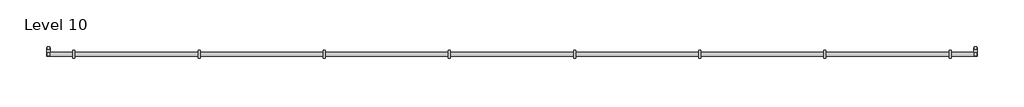
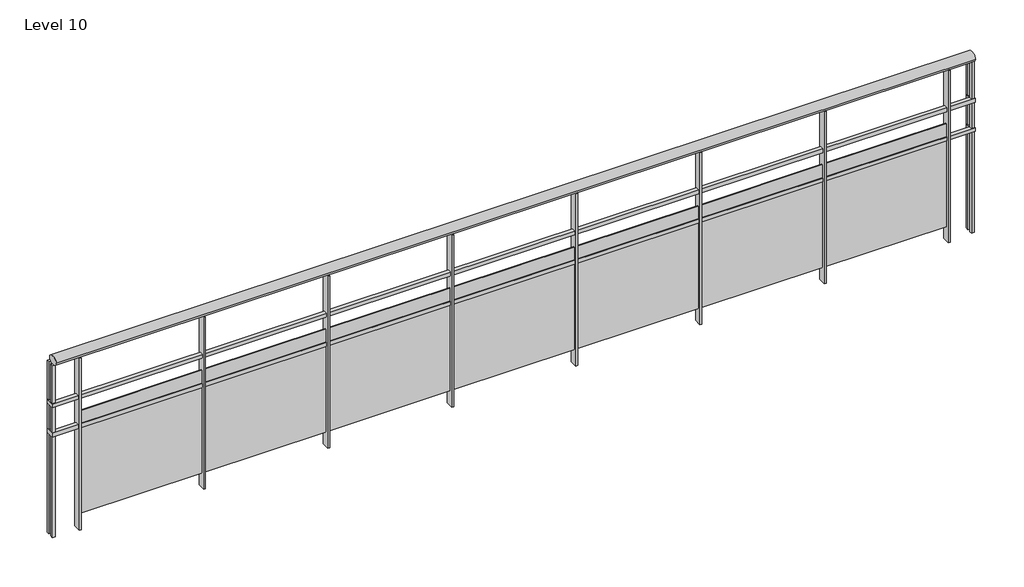
# One storey: 1 railing.
"""IFC4 building model written with IfcOpenShell, lengths in millimetres."""

from ifc_helpers import new_model, si_unit, point, frame, origin, place, context, project, spatial, polyline, ellipse_curve, trimmed, outline, extrude, faceted_brep, element, save
from ifc_brep_helpers import plane_surface, extruded_surface, advanced_brep

model = new_model("IFC4")

# Units and contexts
model_context = context("Model", 3, world=origin())
ifc_project = project(units=[si_unit("LENGTHUNIT", "METRE", prefix="MILLI")], contexts=[model_context])

# Site, building, storey
site = spatial("IfcSite", under=ifc_project)
building = spatial("IfcBuilding", under=site)
storey = spatial("IfcBuildingStorey", under=building, Name="Level 10", Elevation=19812.0)

# Railing
placement = place(None, origin())
element("IfcRailing", 1, ObjectType="Glass Panel - Bottom Fill", at=placement, inside=storey, context=model_context, shape_type="SolidModel", body=[
    advanced_brep(
    [(-17715.2963079, -4526.0757947, 21031.2), (-17715.2963079, -4449.8757947, 21031.2), (-23735.0963079, -4526.0757947, 21031.2), (-23735.0963079, -4449.8757947, 21031.2)],
    [
        (0, 1, ellipse_curve(frame((-17715.2963079, -4487.9757947, 21031.2), z_axis=(1.0, 0.0, 0.0), x_axis=(0.0, 1.0, 0.0)), 38.1, 28.575)),
        (1, 0, ellipse_curve(frame((-17715.2963079, -4487.9757947, 21031.2), z_axis=(1.0, 0.0, 0.0), x_axis=(0.0, 1.0, 0.0)), 38.1, 28.575)),
        (2, 3, ellipse_curve(frame((-23735.0963079, -4487.9757947, 21031.2), z_axis=(-1.0, 0.0, 0.0), x_axis=(0.0, 1.0, 0.0)), 38.1, 28.575)),
        (3, 2, ellipse_curve(frame((-23735.0963079, -4487.9757947, 21031.2), z_axis=(-1.0, 0.0, 0.0), x_axis=(0.0, 1.0, 0.0)), 38.1, 28.575)),
        (0, 2),
        (3, 1),
    ],
    [
        plane_surface(frame((-17715.2963079, -4487.9757947, 21031.2), z_axis=(1.0, 0.0, 0.0), x_axis=(0.0, -1.0, 0.0))),
        plane_surface(frame((-23735.0963079, -4487.9757947, 21031.2), z_axis=(-1.0, 0.0, 0.0), x_axis=(0.0, -1.0, 0.0))),
        extruded_surface(trimmed(ellipse_curve(frame((-23735.0963079, -4487.9757947, 21031.2), z_axis=(1.0, 0.0, 0.0), x_axis=(0.0, 1.0, 0.0)), 38.1, 28.575), [point((-23735.0963079, -4526.0757947, 21031.2))], [point((-23735.0963079, -4449.8757947, 21031.2))], True, "CARTESIAN"), (6019.799999999999, 0.0, 0.0), 6019.799999999999),
        extruded_surface(trimmed(ellipse_curve(frame((-23735.0963079, -4487.9757947, 21031.2), z_axis=(1.0, 0.0, 0.0), x_axis=(0.0, 1.0, 0.0)), 38.1, 28.575), [point((-23735.0963079, -4449.8757947, 21031.2))], [point((-23735.0963079, -4526.0757947, 21031.2))], True, "CARTESIAN"), (6019.799999999999, 0.0, 0.0), 6019.799999999999),
    ],
    [
        (0, [[1, 2]]),
        (1, [[3, 4]]),
        (2, [[-1, 5, -4, 6]]),
        (3, [[-2, -6, -3, -5]]),
    ],
),
    faceted_brep([(-17727.9963079, -4443.5257947, 20739.1), (-17702.5963079, -4443.5257947, 20739.1), (-17702.5963079, -4443.5257947, 20713.7), (-17727.9963079, -4443.5257947, 20713.7), (-17727.9963079, -4475.2757947, 20739.1), (-17702.5963079, -4500.6757947, 20739.1), (-17702.5963079, -4500.6757947, 20713.7), (-17727.9963079, -4475.2757947, 20713.7), (-23722.3963079, -4475.2757947, 20739.1), (-23747.7963079, -4500.6757947, 20739.1), (-23747.7963079, -4500.6757947, 20713.7), (-23722.3963079, -4475.2757947, 20713.7), (-23722.3963079, -4443.5257947, 20739.1), (-23722.3963079, -4443.5257947, 20713.7), (-23747.7963079, -4443.5257947, 20713.7), (-23747.7963079, -4443.5257947, 20739.1)], [[[0, 1, 2, 3]], [[1, 0, 4, 5]], [[2, 1, 5, 6]], [[3, 2, 6, 7]], [[0, 3, 7, 4]], [[5, 4, 8, 9]], [[6, 5, 9, 10]], [[7, 6, 10, 11]], [[4, 7, 11, 8]], [[12, 13, 14, 15]], [[9, 8, 12, 15]], [[10, 9, 15, 14]], [[11, 10, 14, 13]], [[8, 11, 13, 12]]]),
    faceted_brep([(-17727.9963079, -4443.5257947, 20535.9), (-17702.5963079, -4443.5257947, 20535.9), (-17702.5963079, -4443.5257947, 20510.5), (-17727.9963079, -4443.5257947, 20510.5), (-17727.9963079, -4475.2757947, 20535.9), (-17702.5963079, -4500.6757947, 20535.9), (-17702.5963079, -4500.6757947, 20510.5), (-17727.9963079, -4475.2757947, 20510.5), (-23722.3963079, -4475.2757947, 20535.9), (-23747.7963079, -4500.6757947, 20535.9), (-23747.7963079, -4500.6757947, 20510.5), (-23722.3963079, -4475.2757947, 20510.5), (-23722.3963079, -4443.5257947, 20535.9), (-23722.3963079, -4443.5257947, 20510.5), (-23747.7963079, -4443.5257947, 20510.5), (-23747.7963079, -4443.5257947, 20535.9)], [[[0, 1, 2, 3]], [[1, 0, 4, 5]], [[2, 1, 5, 6]], [[3, 2, 6, 7]], [[0, 3, 7, 4]], [[5, 4, 8, 9]], [[6, 5, 9, 10]], [[7, 6, 10, 11]], [[4, 7, 11, 8]], [[12, 13, 14, 15]], [[9, 8, 12, 15]], [[10, 9, 15, 14]], [[11, 10, 14, 13]], [[8, 11, 13, 12]]]),
    extrude(outline(polyline([(-23563.6463079, -4462.5757947), (-23563.6463079, -4513.3757947), (-23576.3463079, -4513.3757947), (-23576.3463079, -4462.5757947), (-23563.6463079, -4462.5757947)])), frame((0.0, 0.0, 19812.0), z_axis=(0.0, 0.0, 1.0), x_axis=(1.0, 0.0, 0.0)), (0.0, 0.0, 1.0), 1190.625),
    extrude(outline(polyline([(-22757.1963079, -4494.5109517), (-23569.9963079, -4494.5109517), (-23569.9963079, -4488.1609517), (-22757.1963079, -4488.1609517), (-22757.1963079, -4494.5109517)])), frame((0.0, 0.0, 19913.6), z_axis=(0.0, 0.0, 1.0), x_axis=(1.0, 0.0, 0.0)), (0.0, 0.0, 1.0), 711.2),
    extrude(outline(polyline([(-22750.8463079, -4462.5757947), (-22750.8463079, -4513.3757947), (-22763.5463079, -4513.3757947), (-22763.5463079, -4462.5757947), (-22750.8463079, -4462.5757947)])), frame((0.0, 0.0, 19812.0), z_axis=(0.0, 0.0, 1.0), x_axis=(1.0, 0.0, 0.0)), (0.0, 0.0, 1.0), 1190.625),
    extrude(outline(polyline([(-21944.3963079, -4494.5109517), (-22757.1963079, -4494.5109517), (-22757.1963079, -4488.1609517), (-21944.3963079, -4488.1609517), (-21944.3963079, -4494.5109517)])), frame((0.0, 0.0, 19913.6), z_axis=(0.0, 0.0, 1.0), x_axis=(1.0, 0.0, 0.0)), (0.0, 0.0, 1.0), 711.2),
    extrude(outline(polyline([(-21938.0463079, -4462.5757947), (-21938.0463079, -4513.3757947), (-21950.7463079, -4513.3757947), (-21950.7463079, -4462.5757947), (-21938.0463079, -4462.5757947)])), frame((0.0, 0.0, 19812.0), z_axis=(0.0, 0.0, 1.0), x_axis=(1.0, 0.0, 0.0)), (0.0, 0.0, 1.0), 1190.625),
    extrude(outline(polyline([(-21131.5963079, -4494.5109517), (-21944.3963079, -4494.5109517), (-21944.3963079, -4488.1609517), (-21131.5963079, -4488.1609517), (-21131.5963079, -4494.5109517)])), frame((0.0, 0.0, 19913.6), z_axis=(0.0, 0.0, 1.0), x_axis=(1.0, 0.0, 0.0)), (0.0, 0.0, 1.0), 711.2),
    extrude(outline(polyline([(-21125.2463079, -4462.5757947), (-21125.2463079, -4513.3757947), (-21137.9463079, -4513.3757947), (-21137.9463079, -4462.5757947), (-21125.2463079, -4462.5757947)])), frame((0.0, 0.0, 19812.0), z_axis=(0.0, 0.0, 1.0), x_axis=(1.0, 0.0, 0.0)), (0.0, 0.0, 1.0), 1190.625),
    extrude(outline(polyline([(-20318.7963079, -4494.5109517), (-21131.5963079, -4494.5109517), (-21131.5963079, -4488.1609517), (-20318.7963079, -4488.1609517), (-20318.7963079, -4494.5109517)])), frame((0.0, 0.0, 19913.6), z_axis=(0.0, 0.0, 1.0), x_axis=(1.0, 0.0, 0.0)), (0.0, 0.0, 1.0), 711.2),
    extrude(outline(polyline([(-20312.4463079, -4462.5757947), (-20312.4463079, -4513.3757947), (-20325.1463079, -4513.3757947), (-20325.1463079, -4462.5757947), (-20312.4463079, -4462.5757947)])), frame((0.0, 0.0, 19812.0), z_axis=(0.0, 0.0, 1.0), x_axis=(1.0, 0.0, 0.0)), (0.0, 0.0, 1.0), 1190.625),
    extrude(outline(polyline([(-19505.9963079, -4494.5109517), (-20318.7963079, -4494.5109517), (-20318.7963079, -4488.1609517), (-19505.9963079, -4488.1609517), (-19505.9963079, -4494.5109517)])), frame((0.0, 0.0, 19913.6), z_axis=(0.0, 0.0, 1.0), x_axis=(1.0, 0.0, 0.0)), (0.0, 0.0, 1.0), 711.2),
    extrude(outline(polyline([(-19499.6463079, -4462.5757947), (-19499.6463079, -4513.3757947), (-19512.3463079, -4513.3757947), (-19512.3463079, -4462.5757947), (-19499.6463079, -4462.5757947)])), frame((0.0, 0.0, 19812.0), z_axis=(0.0, 0.0, 1.0), x_axis=(1.0, 0.0, 0.0)), (0.0, 0.0, 1.0), 1190.625),
    extrude(outline(polyline([(-18693.1963079, -4494.5109517), (-19505.9963079, -4494.5109517), (-19505.9963079, -4488.1609517), (-18693.1963079, -4488.1609517), (-18693.1963079, -4494.5109517)])), frame((0.0, 0.0, 19913.6), z_axis=(0.0, 0.0, 1.0), x_axis=(1.0, 0.0, 0.0)), (0.0, 0.0, 1.0), 711.2),
    extrude(outline(polyline([(-18686.8463079, -4462.5757947), (-18686.8463079, -4513.3757947), (-18699.5463079, -4513.3757947), (-18699.5463079, -4462.5757947), (-18686.8463079, -4462.5757947)])), frame((0.0, 0.0, 19812.0), z_axis=(0.0, 0.0, 1.0), x_axis=(1.0, 0.0, 0.0)), (0.0, 0.0, 1.0), 1190.625),
    extrude(outline(polyline([(-17880.3963079, -4494.5109517), (-18693.1963079, -4494.5109517), (-18693.1963079, -4488.1609517), (-17880.3963079, -4488.1609517), (-17880.3963079, -4494.5109517)])), frame((0.0, 0.0, 19913.6), z_axis=(0.0, 0.0, 1.0), x_axis=(1.0, 0.0, 0.0)), (0.0, 0.0, 1.0), 711.2),
    extrude(outline(polyline([(-17874.0463079, -4462.5757947), (-17874.0463079, -4513.3757947), (-17886.7463079, -4513.3757947), (-17886.7463079, -4462.5757947), (-17874.0463079, -4462.5757947)])), frame((0.0, 0.0, 19812.0), z_axis=(0.0, 0.0, 1.0), x_axis=(1.0, 0.0, 0.0)), (0.0, 0.0, 1.0), 1190.625),
    extrude(outline(polyline([(-23725.5713079, -4478.4507947), (-23725.5713079, -4497.5007947), (-23744.6213079, -4497.5007947), (-23744.6213079, -4478.4507947), (-23725.5713079, -4478.4507947)])), frame((0.0, 0.0, 19812.0), z_axis=(0.0, 0.0, 1.0), x_axis=(1.0, 0.0, 0.0)), (0.0, 0.0, 1.0), 1190.625),
    extrude(outline(polyline([(-17724.8213079, -4478.4507947), (-17705.7713079, -4478.4507947), (-17705.7713079, -4497.5007947), (-17724.8213079, -4497.5007947), (-17724.8213079, -4478.4507947)])), frame((0.0, 0.0, 19812.0), z_axis=(0.0, 0.0, 1.0), x_axis=(1.0, 0.0, 0.0)), (0.0, 0.0, 1.0), 1190.625),
    extrude(outline(polyline([(-23725.5713079, -4456.2257947), (-23744.6213079, -4456.2257947), (-23744.6213079, -4437.1757947), (-23725.5713079, -4437.1757947), (-23725.5713079, -4456.2257947)])), frame((0.0, 0.0, 19812.0), z_axis=(0.0, 0.0, 1.0), x_axis=(1.0, 0.0, 0.0)), (0.0, 0.0, 1.0), 1190.625),
    extrude(outline(polyline([(-17724.8213079, -4437.1757947), (-17705.7713079, -4437.1757947), (-17705.7713079, -4456.2257947), (-17724.8213079, -4456.2257947), (-17724.8213079, -4437.1757947)])), frame((0.0, 0.0, 19812.0), z_axis=(0.0, 0.0, 1.0), x_axis=(1.0, 0.0, 0.0)), (0.0, 0.0, 1.0), 1190.625),
])

save(model, "model.ifc")

# Revit data of these elements
# Type "Glass Panel - Bottom Fill"
#   Assembly Code = "C2010400"
#   built-in parameter 1008612 = 0.0416667 (stored number, unit not read)
#   built-in parameter 1008611 = 0.0416667 (stored number, unit not read)
#   built-in parameter 1008609 = 0.333333 (stored number, unit not read)
#   built-in parameter 1008604 = 0.166667 (stored number, unit not read)
#   built-in parameter 1008603 = 0.166667 (stored number, unit not read)
#   Railing Height = 4' - 0"
#   built-in parameter 1008630 = 2
#   built-in parameter 1008610 = 2
#   built-in parameter 1008618 = Baluster - Square : 3/4"
# Element 1 (IfcRailing, "Glass Panel - Bottom Fill")
#   Phase Created = New Construction
#   Materials on its faces: "Glass"
# Materials
#   "Glass": class "Glass", colour RGB 218 227 224, transparency 0.85, Description = "Soda Lime Glass", Cost = 0
